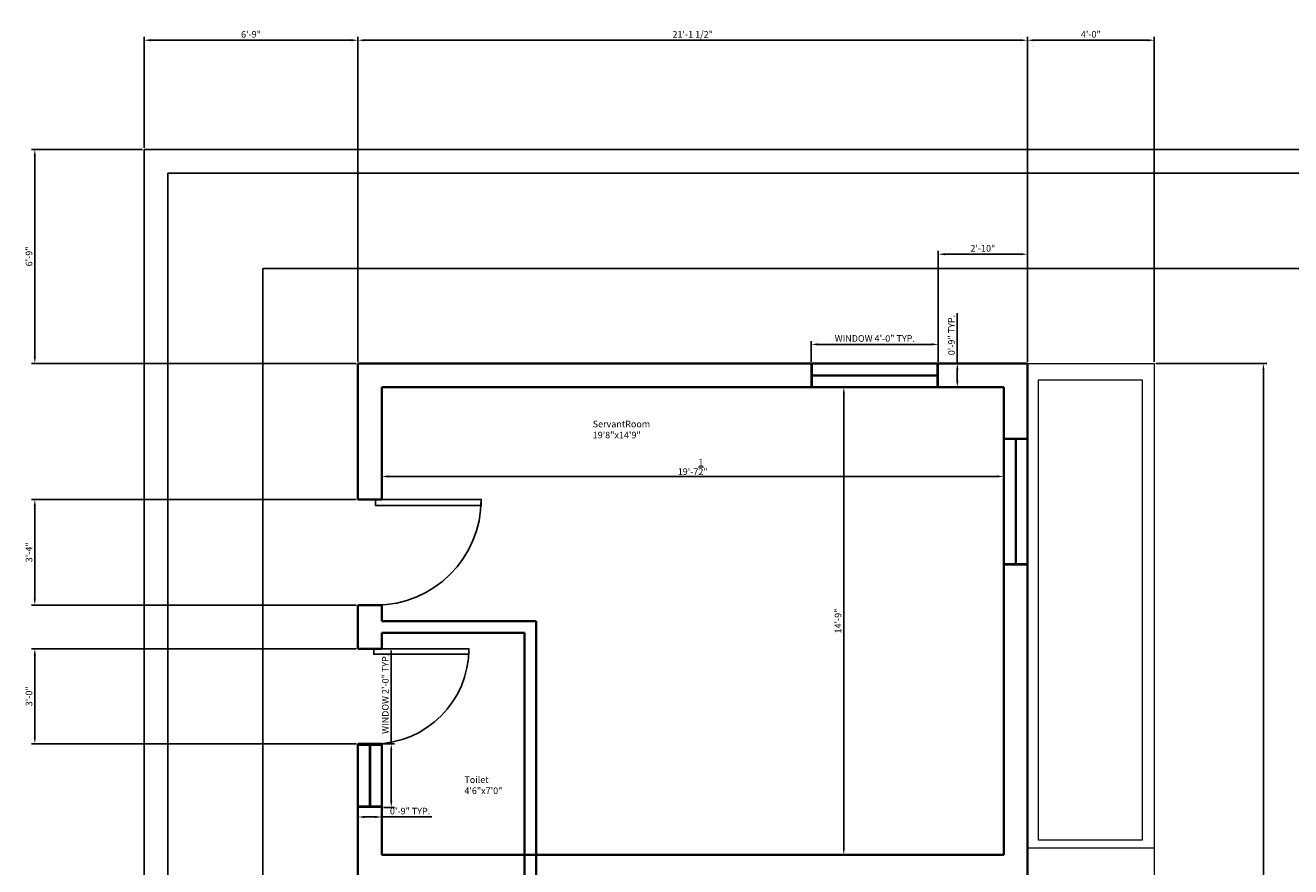
# Model space of a CAD drawing. Units: inches. Extents: x 250205121 to 250208111, y 89832590 to 89833271.
# Tile 2 of 14: x 250205121 to 250205601, y 89832953 to 89833271. Entities that reach past the tile are written whole.
import ezdxf

# ---------------------------------------------------------------- set-up
doc = ezdxf.new("R2010")
doc.units = ezdxf.units.IN
for name, color, linetype, lineweight in [('A-AREA-IDEN', 4, 'Continuous', 18), ('A-FLOR', 7, 'Continuous', 18), ('A-WALL', 7, 'Continuous', 35), ('C-PROP', 8, 'Continuous', 25), ('dimensions', 2, 'Continuous', 18), ('doors', 3, 'Continuous', 25), ('window', 4, 'Continuous', 18)]:
    doc.layers.add(name, color=color, linetype=linetype, lineweight=lineweight)
doc.styles.get("Standard").update_dxf_attribs({"font": 'arial.ttf'})
doc.dimstyles.new('ISO-25', dxfattribs={"dimtxt": 2.5, "dimasz": 2.5, "dimexe": 1.25, "dimexo": 0.625, "dimtad": 1, "dimlunit": 4, "dimtxsty": 'Standard', "dimcen": 2.5, "dimadec": 0, "dimazin": 0, "dimtfac": 1, "dimtmove": 0, "dimatfit": 3, "dimfxl": 1, "dimarcsym": 0})

# ---------------------------------------------------------------- blocks, each defined once
blk = doc.blocks.new('*U2')
for p, q in [((0, 0), (0, -5)), ((30, 0), (30, -5))]:
    blk.add_line(p, q)
blk.add_lwpolyline([(0, 0), (0, 30), (1.75, 30), (1.75, 0)], close=True)
blk.add_arc((0, 0), 30, 0, 90)
blk = doc.blocks.new('*D3')
at = {"layer": 'Defpoints', "color": 0, "transparency": 16777216}
for p in [(250205406.37, 89833134.33), (250205406.37, 89832957.33), (250205431.38, 89832957.33)]:
    blk.add_point(p, dxfattribs=at)
at = {"layer": 'dimensions', "color": 0, "lineweight": -2, "transparency": 16777216}
for p, q in [((250205406.99, 89833134.33), (250205432.63, 89833134.33)), ((250205431.38, 89833131.83), (250205431.38, 89832959.83)), ((250205406.99, 89832957.33), (250205432.63, 89832957.33))]:
    blk.add_line(p, q, dxfattribs=at)
at = {"layer": 'dimensions', "color": 0, "transparency": 16777216}
for points in [[(250205430.97, 89833131.83), (250205431.8, 89833131.83), (250205431.38, 89833134.33)], [(250205430.97, 89832959.83), (250205431.8, 89832959.83), (250205431.38, 89832957.33)]]:
    blk.add_solid(points, dxfattribs=at)
at = {"layer": 'dimensions', "color": 0, "transparency": 16777216, "insert": (250205429.48, 89833045.83), "char_height": 2.5, "attachment_point": 5, "rotation": 90}
blk.add_mtext('14\'-9"', dxfattribs=at)
blk = doc.blocks.new('*D4')
at = {"layer": 'Defpoints', "color": 0, "transparency": 16777216}
for p in [(250205256.41, 89833120.81), (250205491.91, 89833120.81), (250205491.91, 89833100.55)]:
    blk.add_point(p, dxfattribs=at)
at = {"layer": 'dimensions', "color": 0, "lineweight": -2, "transparency": 16777216}
for p, q in [((250205256.41, 89833120.18), (250205256.41, 89833099.3)), ((250205491.91, 89833120.18), (250205491.91, 89833099.3)), ((250205258.91, 89833100.55), (250205489.41, 89833100.55))]:
    blk.add_line(p, q, dxfattribs=at)
at = {"layer": 'dimensions', "color": 0, "transparency": 16777216}
for points in [[(250205258.91, 89833100.97), (250205258.91, 89833100.14), (250205256.41, 89833100.55)], [(250205489.41, 89833100.97), (250205489.41, 89833100.14), (250205491.91, 89833100.55)]]:
    blk.add_solid(points, dxfattribs=at)
at = {"layer": 'dimensions', "color": 0, "transparency": 16777216, "insert": (250205374.16, 89833104.13), "char_height": 2.5, "attachment_point": 5}
blk.add_mtext('19\'-7{\\H1x;\\S1/2;}"', dxfattribs=at)
blk = doc.blocks.new('WIN-24IN')
for p, q in [((0, 0), (0, 24.08)), ((0, 24.08), (9, 24.08)), ((9, 24.08), (9, 0)), ((0, 23.58), (9, 23.58)), ((4.3, 23.58), (4.3, 0.5)), ((4.7, 23.58), (4.7, 0.5)), ((9, 0.5), (0, 0.5)), ((9, 0), (0, 0))]:
    blk.add_line(p, q)
blk = doc.blocks.new('WIN-48IN')
for p, q in [((0, 0), (0, 48.08)), ((0, 48.08), (9, 48.08)), ((9, 48.08), (9, 0)), ((0, 47.58), (9, 47.58)), ((4.3, 47.58), (4.3, 0.5)), ((4.7, 47.58), (4.7, 0.5)), ((9, 0.5), (0, 0.5)), ((9, 0), (0, 0))]:
    blk.add_line(p, q)
blk = doc.blocks.new('*D29')
at = {"layer": 'Defpoints', "color": 0, "transparency": 16777216}
for p in [(250205256.41, 89832999.33), (250205260.02, 89832999.33), (250205256.41, 89832975.25)]:
    blk.add_point(p, dxfattribs=at)
at = {"layer": 'dimensions', "color": 0, "lineweight": -2, "transparency": 16777216}
for p, q in [((250205260.02, 89832999.33), (250205260.02, 89833034.71)), ((250205257.03, 89832999.33), (250205261.27, 89832999.33)), ((250205260.02, 89832977.75), (250205260.02, 89832996.83)), ((250205257.03, 89832975.25), (250205261.27, 89832975.25))]:
    blk.add_line(p, q, dxfattribs=at)
at = {"layer": 'dimensions', "color": 0, "transparency": 16777216}
for points in [[(250205259.6, 89832996.83), (250205260.44, 89832996.83), (250205260.02, 89832999.33)], [(250205259.6, 89832977.75), (250205260.44, 89832977.75), (250205260.02, 89832975.25)]]:
    blk.add_solid(points, dxfattribs=at)
at = {"layer": 'dimensions', "color": 0, "transparency": 16777216, "insert": (250205258.1, 89833018.27), "char_height": 2.5, "attachment_point": 5, "rotation": 90}
blk.add_mtext('WINDOW 2\'-0" TYP.', dxfattribs=at)
blk = doc.blocks.new('*D30')
at = {"layer": 'Defpoints', "color": 0, "transparency": 16777216}
for p in [(250205247.41, 89832975.25), (250205256.41, 89832975.25), (250205256.41, 89832971.64)]:
    blk.add_point(p, dxfattribs=at)
at = {"layer": 'dimensions', "color": 0, "lineweight": -2, "transparency": 16777216}
for p, q in [((250205247.41, 89832974.62), (250205247.41, 89832970.39)), ((250205256.41, 89832974.62), (250205256.41, 89832970.39)), ((250205249.91, 89832971.64), (250205253.91, 89832971.64)), ((250205256.41, 89832971.64), (250205275.4, 89832971.64))]:
    blk.add_line(p, q, dxfattribs=at)
at = {"layer": 'dimensions', "color": 0, "transparency": 16777216}
for points in [[(250205249.91, 89832972.05), (250205249.91, 89832971.22), (250205247.41, 89832971.64)], [(250205253.91, 89832972.05), (250205253.91, 89832971.22), (250205256.41, 89832971.64)]]:
    blk.add_solid(points, dxfattribs=at)
at = {"layer": 'dimensions', "color": 0, "transparency": 16777216, "insert": (250205267.15, 89832973.54), "char_height": 2.5, "attachment_point": 5}
blk.add_mtext('0\'-9" TYP.', dxfattribs=at)
blk = doc.blocks.new('*D31')
at = {"layer": 'Defpoints', "color": 0, "transparency": 16777216}
for p in [(250205419.07, 89833150.54), (250205419.07, 89833143.33), (250205467.15, 89833143.33)]:
    blk.add_point(p, dxfattribs=at)
at = {"layer": 'dimensions', "color": 0, "lineweight": -2, "transparency": 16777216}
for p, q in [((250205419.07, 89833143.95), (250205419.07, 89833151.79)), ((250205467.15, 89833143.95), (250205467.15, 89833151.79)), ((250205464.65, 89833150.54), (250205421.57, 89833150.54))]:
    blk.add_line(p, q, dxfattribs=at)
at = {"layer": 'dimensions', "color": 0, "transparency": 16777216}
for points in [[(250205421.57, 89833150.96), (250205421.57, 89833150.12), (250205419.07, 89833150.54)], [(250205464.65, 89833150.96), (250205464.65, 89833150.12), (250205467.15, 89833150.54)]]:
    blk.add_solid(points, dxfattribs=at)
at = {"layer": 'dimensions', "color": 0, "transparency": 16777216, "insert": (250205443.11, 89833152.46), "char_height": 2.5, "attachment_point": 5, "rotation": 0}
blk.add_mtext('WINDOW 4\'-0" TYP.', dxfattribs=at)
blk = doc.blocks.new('*D32')
at = {"layer": 'Defpoints', "color": 0, "transparency": 16777216}
for p in [(250205467.15, 89833143.33), (250205474.36, 89833143.33), (250205467.15, 89833134.33)]:
    blk.add_point(p, dxfattribs=at)
at = {"layer": 'dimensions', "color": 0, "lineweight": -2, "transparency": 16777216}
for p, q in [((250205474.36, 89833143.33), (250205474.36, 89833162.32)), ((250205467.77, 89833143.33), (250205475.61, 89833143.33)), ((250205474.36, 89833136.83), (250205474.36, 89833140.83)), ((250205467.77, 89833134.33), (250205475.61, 89833134.33))]:
    blk.add_line(p, q, dxfattribs=at)
at = {"layer": 'dimensions', "color": 0, "transparency": 16777216}
for points in [[(250205473.94, 89833140.83), (250205474.78, 89833140.83), (250205474.36, 89833143.33)], [(250205473.94, 89833136.83), (250205474.78, 89833136.83), (250205474.36, 89833134.33)]]:
    blk.add_solid(points, dxfattribs=at)
at = {"layer": 'dimensions', "color": 0, "transparency": 16777216, "insert": (250205472.46, 89833154.07), "char_height": 2.5, "attachment_point": 5, "rotation": 90}
blk.add_mtext('0\'-9" TYP.', dxfattribs=at)
blk = doc.blocks.new('*D43')
at = {"layer": 'Defpoints', "color": 0, "transparency": 16777216}
for p in [(250205247.41, 89833265.68), (250205166.41, 89833224.33), (250205247.41, 89833143.33)]:
    blk.add_point(p, dxfattribs=at)
at = {"layer": 'dimensions', "color": 0, "lineweight": -2, "transparency": 16777216}
for p, q in [((250205166.41, 89833224.95), (250205166.41, 89833266.93)), ((250205247.41, 89833143.95), (250205247.41, 89833266.93)), ((250205168.91, 89833265.68), (250205244.91, 89833265.68))]:
    blk.add_line(p, q, dxfattribs=at)
at = {"layer": 'dimensions', "color": 0, "transparency": 16777216}
for points in [[(250205168.91, 89833266.09), (250205168.91, 89833265.26), (250205166.41, 89833265.68)], [(250205244.91, 89833266.09), (250205244.91, 89833265.26), (250205247.41, 89833265.68)]]:
    blk.add_solid(points, dxfattribs=at)
at = {"layer": 'dimensions', "color": 0, "transparency": 16777216, "insert": (250205206.91, 89833267.58), "char_height": 2.5, "attachment_point": 5}
blk.add_mtext('6\'-9"', dxfattribs=at)
blk = doc.blocks.new('*D44')
at = {"layer": 'Defpoints', "color": 0, "transparency": 16777216}
for p in [(250205125.06, 89833224.33), (250205166.41, 89833224.33), (250205247.41, 89833143.33)]:
    blk.add_point(p, dxfattribs=at)
at = {"layer": 'dimensions', "color": 0, "lineweight": -2, "transparency": 16777216}
for p, q in [((250205165.78, 89833224.33), (250205123.81, 89833224.33)), ((250205125.06, 89833145.83), (250205125.06, 89833221.83)), ((250205246.78, 89833143.33), (250205123.81, 89833143.33))]:
    blk.add_line(p, q, dxfattribs=at)
at = {"layer": 'dimensions', "color": 0, "transparency": 16777216}
for points in [[(250205124.64, 89833221.83), (250205125.47, 89833221.83), (250205125.06, 89833224.33)], [(250205124.64, 89833145.83), (250205125.47, 89833145.83), (250205125.06, 89833143.33)]]:
    blk.add_solid(points, dxfattribs=at)
at = {"layer": 'dimensions', "color": 0, "transparency": 16777216, "insert": (250205123.16, 89833183.83), "char_height": 2.5, "attachment_point": 5, "rotation": 90}
blk.add_mtext('6\'-9"', dxfattribs=at)
blk = doc.blocks.new('*D45')
at = {"layer": 'Defpoints', "color": 0, "transparency": 16777216}
for p in [(250205500.91, 89833265.68), (250205247.41, 89833143.33), (250205500.91, 89833143.33)]:
    blk.add_point(p, dxfattribs=at)
at = {"layer": 'dimensions', "color": 0, "lineweight": -2, "transparency": 16777216}
for p, q in [((250205247.41, 89833143.95), (250205247.41, 89833266.93)), ((250205500.91, 89833143.95), (250205500.91, 89833266.93)), ((250205249.91, 89833265.68), (250205498.41, 89833265.68))]:
    blk.add_line(p, q, dxfattribs=at)
at = {"layer": 'dimensions', "color": 0, "transparency": 16777216}
for points in [[(250205249.91, 89833266.09), (250205249.91, 89833265.26), (250205247.41, 89833265.68)], [(250205498.41, 89833266.09), (250205498.41, 89833265.26), (250205500.91, 89833265.68)]]:
    blk.add_solid(points, dxfattribs=at)
at = {"layer": 'dimensions', "color": 0, "transparency": 16777216, "insert": (250205374.16, 89833267.6), "char_height": 2.5, "attachment_point": 5}
blk.add_mtext('21\'-1 1/2"', dxfattribs=at)
blk = doc.blocks.new('*D46')
at = {"layer": 'Defpoints', "color": 0, "transparency": 16777216}
for p in [(250205548.91, 89833265.68), (250205500.91, 89833143.33), (250205548.91, 89833143.33)]:
    blk.add_point(p, dxfattribs=at)
at = {"layer": 'dimensions', "color": 0, "lineweight": -2, "transparency": 16777216}
for p, q in [((250205500.91, 89833143.95), (250205500.91, 89833266.93)), ((250205548.91, 89833143.95), (250205548.91, 89833266.93)), ((250205503.41, 89833265.68), (250205546.41, 89833265.68))]:
    blk.add_line(p, q, dxfattribs=at)
at = {"layer": 'dimensions', "color": 0, "transparency": 16777216}
for points in [[(250205503.41, 89833266.09), (250205503.41, 89833265.26), (250205500.91, 89833265.68)], [(250205546.41, 89833266.09), (250205546.41, 89833265.26), (250205548.91, 89833265.68)]]:
    blk.add_solid(points, dxfattribs=at)
at = {"layer": 'dimensions', "color": 0, "transparency": 16777216, "insert": (250205524.91, 89833267.58), "char_height": 2.5, "attachment_point": 5}
blk.add_mtext('4\'-0"', dxfattribs=at)
blk = doc.blocks.new('*D48')
at = {"layer": 'Defpoints', "color": 0, "transparency": 16777216}
for p in [(250205548.91, 89833143.33), (250205548.91, 89832714.33), (250205590.26, 89832714.33)]:
    blk.add_point(p, dxfattribs=at)
at = {"layer": 'dimensions', "color": 0, "lineweight": -2, "transparency": 16777216}
for p, q in [((250205549.53, 89833143.33), (250205591.51, 89833143.33)), ((250205590.26, 89833140.83), (250205590.26, 89832716.83)), ((250205549.53, 89832714.33), (250205591.51, 89832714.33))]:
    blk.add_line(p, q, dxfattribs=at)
at = {"layer": 'dimensions', "color": 0, "transparency": 16777216}
for points in [[(250205589.84, 89833140.83), (250205590.67, 89833140.83), (250205590.26, 89833143.33)], [(250205589.84, 89832716.83), (250205590.67, 89832716.83), (250205590.26, 89832714.33)]]:
    blk.add_solid(points, dxfattribs=at)
at = {"layer": 'dimensions', "color": 0, "transparency": 16777216, "insert": (250205588.36, 89832928.83), "char_height": 2.5, "attachment_point": 5, "rotation": 90}
blk.add_mtext('35\'-9"', dxfattribs=at)
blk = doc.blocks.new('*D50')
at = {"layer": 'Defpoints', "color": 0, "transparency": 16777216}
for p in [(250205125.06, 89833091.83), (250205247.41, 89833091.83), (250205247.41, 89833051.83)]:
    blk.add_point(p, dxfattribs=at)
at = {"layer": 'dimensions', "color": 0, "lineweight": -2, "transparency": 16777216}
for p, q in [((250205246.78, 89833091.83), (250205123.81, 89833091.83)), ((250205125.06, 89833054.33), (250205125.06, 89833089.33)), ((250205246.78, 89833051.83), (250205123.81, 89833051.83))]:
    blk.add_line(p, q, dxfattribs=at)
at = {"layer": 'dimensions', "color": 0, "transparency": 16777216}
for points in [[(250205124.64, 89833089.33), (250205125.47, 89833089.33), (250205125.06, 89833091.83)], [(250205124.64, 89833054.33), (250205125.47, 89833054.33), (250205125.06, 89833051.83)]]:
    blk.add_solid(points, dxfattribs=at)
at = {"layer": 'dimensions', "color": 0, "transparency": 16777216, "insert": (250205123.16, 89833071.83), "char_height": 2.5, "attachment_point": 5, "rotation": 90}
blk.add_mtext('3\'-4"', dxfattribs=at)
blk = doc.blocks.new('*D51')
at = {"layer": 'Defpoints', "color": 0, "transparency": 16777216}
for p in [(250205125.06, 89833035.33), (250205247.41, 89833035.33), (250205247.41, 89832999.33)]:
    blk.add_point(p, dxfattribs=at)
at = {"layer": 'dimensions', "color": 0, "lineweight": -2, "transparency": 16777216}
for p, q in [((250205246.78, 89833035.33), (250205123.81, 89833035.33)), ((250205125.06, 89833001.83), (250205125.06, 89833032.83)), ((250205246.78, 89832999.33), (250205123.81, 89832999.33))]:
    blk.add_line(p, q, dxfattribs=at)
at = {"layer": 'dimensions', "color": 0, "transparency": 16777216}
for points in [[(250205124.64, 89833032.83), (250205125.47, 89833032.83), (250205125.06, 89833035.33)], [(250205124.64, 89833001.83), (250205125.47, 89833001.83), (250205125.06, 89832999.33)]]:
    blk.add_solid(points, dxfattribs=at)
at = {"layer": 'dimensions', "color": 0, "transparency": 16777216, "insert": (250205123.16, 89833017.33), "char_height": 2.5, "attachment_point": 5, "rotation": 90}
blk.add_mtext('3\'-0"', dxfattribs=at)
blk = doc.blocks.new('*D53')
at = {"layer": 'Defpoints', "color": 0, "transparency": 16777216}
for p in [(250205500.91, 89833184.68), (250205467.15, 89833143.33), (250205500.91, 89833143.33)]:
    blk.add_point(p, dxfattribs=at)
at = {"layer": 'dimensions', "color": 0, "lineweight": -2, "transparency": 16777216}
for p, q in [((250205467.15, 89833143.95), (250205467.15, 89833185.93)), ((250205469.65, 89833184.68), (250205498.41, 89833184.68)), ((250205500.91, 89833143.95), (250205500.91, 89833185.93))]:
    blk.add_line(p, q, dxfattribs=at)
at = {"layer": 'dimensions', "color": 0, "transparency": 16777216}
for points in [[(250205469.65, 89833185.09), (250205469.65, 89833184.26), (250205467.15, 89833184.68)], [(250205498.41, 89833185.09), (250205498.41, 89833184.26), (250205500.91, 89833184.68)]]:
    blk.add_solid(points, dxfattribs=at)
at = {"layer": 'dimensions', "color": 0, "transparency": 16777216, "insert": (250205484.03, 89833186.58), "char_height": 2.5, "attachment_point": 5}
blk.add_mtext('2\'-10"', dxfattribs=at)

msp = doc.modelspace()

# ---------------------------------------------------------------- linework, layer by layer
at = {"layer": 'A-FLOR'}
for p, q in [((250205500.908, 89833143.328), (250205524.908, 89833143.328)), ((250205524.908, 89833143.328), (250205548.908, 89833143.328)), ((250205548.908, 89833143.328), (250205548.908, 89832714.328)), ((250205500.908, 89832959.99), (250205548.908, 89832959.99))]:
    msp.add_line(p, q, dxfattribs=at)
msp.add_lwpolyline([(250205505.113, 89833137.184), (250205544.324, 89833137.184), (250205544.324, 89832962.894), (250205505.113, 89832962.894)], close=True, dxfattribs=at)
at = {"layer": 'A-WALL'}
for p, q in [((250205256.408, 89833143.328), (250205247.408, 89833143.328)), ((250205247.408, 89833143.328), (250205247.408, 89833134.328)), ((250205500.908, 89833143.328), (250205256.408, 89833143.328)), ((250205500.908, 89833134.328), (250205500.908, 89833143.328)), ((250205247.408, 89833134.328), (250205247.408, 89833091.828)), ((250205256.408, 89833134.328), (250205491.908, 89833134.328)), ((250205256.408, 89833134.328), (250205256.408, 89833091.828)), ((250205491.908, 89832957.328), (250205491.908, 89833134.328)), ((250205500.908, 89832948.328), (250205500.908, 89833134.328)), ((250205247.408, 89833091.828), (250205256.408, 89833091.828)), ((250205256.408, 89833051.828), (250205247.408, 89833051.828)), ((250205247.408, 89833051.828), (250205247.408, 89833035.328)), ((250205256.408, 89833045.828), (250205256.408, 89833051.828)), ((250205256.408, 89833051.828), (250205256.408, 89833045.828)), ((250205256.408, 89833045.828), (250205314.908, 89833045.828)), ((250205314.908, 89833045.828), (250205314.908, 89832888.328)), ((250205256.408, 89833041.328), (250205310.408, 89833041.328)), ((250205256.408, 89833041.328), (250205256.408, 89833035.328)), ((250205256.408, 89833041.328), (250205256.408, 89833035.328)), ((250205310.408, 89833041.328), (250205310.408, 89832888.328)), ((250205256.408, 89833035.328), (250205247.408, 89833035.328)), ((250205247.408, 89832999.328), (250205256.408, 89832999.328)), ((250205247.408, 89832999.328), (250205247.408, 89832948.328)), ((250205256.408, 89832999.328), (250205256.408, 89832957.328)), ((250205256.408, 89832957.328), (250205491.908, 89832957.328))]:
    msp.add_line(p, q, dxfattribs=at)
at = {"layer": 'C-PROP'}
for p, q in [((250205166.408, 89833224.328), (250205166.408, 89832633.328)), ((250205500.908, 89833224.328), (250205166.408, 89833224.328)), ((250205500.908, 89833224.328), (250205977.908, 89833224.328)), ((250205500.908, 89833215.328), (250205175.408, 89833215.328)), ((250205175.408, 89833215.328), (250205175.408, 89832642.328)), ((250205977.908, 89833215.328), (250205500.908, 89833215.328)), ((250205500.908, 89833179.328), (250205211.408, 89833179.328)), ((250205211.408, 89833179.328), (250205211.408, 89832678.328)), ((250205500.908, 89833179.328), (250205509.908, 89833179.328)), ((250205509.908, 89833179.328), (250205680.908, 89833179.328))]:
    msp.add_line(p, q, dxfattribs=at)

# ---------------------------------------------------------------- block references
at = {"layer": 'doors', "rotation": 270}
for p, xscale, yscale, zscale in [((250205254.074, 89833091.828), 1.333333333333333, 1.333333333333333, 1.333333333333333), ((250205253.408, 89833035.328), 1.199999999999999, 1.199999999999999, 1.199999999999999)]:
    msp.add_blockref('*U2', p, dxfattribs=dict(at, xscale=xscale, yscale=yscale, zscale=zscale))
at = {"layer": 'window', "rotation": 90.00000004715952}
msp.add_blockref('WIN-48IN', (250205467.149, 89833134.328), dxfattribs=at)
at = {"layer": 'window'}
for name, p in [('WIN-48IN', (250205491.908, 89833067.021)), ('WIN-24IN', (250205247.408, 89832975.249))]:
    msp.add_blockref(name, p, dxfattribs=at)

# ---------------------------------------------------------------- texts
at = {"layer": 'A-AREA-IDEN', "char_height": 2.5, "attachment_point": 1}
for s, insert in [('ServantRoom\\P19\'8"x14\'9"', (250205336.292, 89833121.638)), ('Toilet\\P4\'6"x7\'0"', (250205287.708, 89832986.993))]:
    msp.add_mtext_dynamic_manual_height_columns(s, width=2.73747, gutter_width=12.5, heights=[0], dxfattribs=dict(at, insert=insert))

# ---------------------------------------------------------------- dimensions: what is measured, and where the dimension line sits
at = {"layer": 'dimensions'}
for base, p1, p2, override, picture, middle in [((250205500.908, 89833265.678), (250205247.408, 89833143.328), (250205500.908, 89833143.328), {"dimdec": 1, "dimlfac": 1, "dimrnd": 0, "dimzin": 1, "dimdsep": 46, "dimlunit": 4, "dimfrac": 2}, '*D45', (250205374.158, 89833267.596)), ((250205247.408, 89833265.678), (250205166.408, 89833224.328), (250205247.408, 89833143.328), {"dimdec": 1, "dimlfac": 1, "dimrnd": 0, "dimzin": 1, "dimdsep": 46, "dimlunit": 4, "dimfrac": 2}, '*D43', (250205206.908, 89833267.579)), ((250205548.908, 89833265.678), (250205500.908, 89833143.328), (250205548.908, 89833143.328), {"dimdec": 1, "dimlfac": 1, "dimrnd": 0, "dimzin": 1, "dimdsep": 46, "dimlunit": 4, "dimfrac": 2}, '*D46', (250205524.908, 89833267.579)), ((250205491.908, 89833100.553), (250205256.408, 89833120.808), (250205491.908, 89833120.808), {"dimclrd": 0, "dimclre": 0, "dimclrt": 0}, '*D4', (250205374.158, 89833104.126))]:
    dim = msp.add_linear_dim(base=base, p1=p1, p2=p2, dimstyle='ISO-25', override=override, dxfattribs=at)
    dim.commit()
    dim.dimension.update_dxf_attribs({"geometry": picture, "text_midpoint": middle})
for base, p1, p2, angle, override, picture, middle in [((250205125.058, 89833224.328), (250205247.408, 89833143.328), (250205166.408, 89833224.328), 90, {"dimdec": 1, "dimlfac": 1, "dimrnd": 0, "dimzin": 1, "dimdsep": 46, "dimlunit": 4, "dimfrac": 2}, '*D44', (250205123.156, 89833183.828)), ((250205500.908, 89833184.678), (250205467.149, 89833143.328), (250205500.908, 89833143.328), 360, {"dimdec": 1, "dimlfac": 1, "dimrnd": 0, "dimzin": 1, "dimdsep": 46, "dimlunit": 4, "dimfrac": 2}, '*D53', (250205484.029, 89833186.579)), ((250205590.258, 89832714.328), (250205548.908, 89833143.328), (250205548.908, 89832714.328), 270, {"dimdec": 1, "dimlfac": 1, "dimrnd": 0, "dimzin": 1, "dimdsep": 46, "dimlunit": 4, "dimfrac": 2}, '*D48', (250205588.355, 89832928.828)), ((250205431.382, 89832957.328), (250205406.369, 89833134.328), (250205406.369, 89832957.328), 90, {"dimclrd": 0, "dimclre": 0, "dimclrt": 0}, '*D3', (250205429.481, 89833045.828)), ((250205125.058, 89833091.828), (250205247.408, 89833051.828), (250205247.408, 89833091.828), 90, {"dimdec": 1, "dimlfac": 1, "dimrnd": 0, "dimzin": 1, "dimdsep": 46, "dimlunit": 4, "dimfrac": 2}, '*D50', (250205123.155, 89833071.828)), ((250205125.058, 89833035.328), (250205247.408, 89832999.328), (250205247.408, 89833035.328), 90, {"dimdec": 1, "dimlfac": 1, "dimrnd": 0, "dimzin": 1, "dimdsep": 46, "dimlunit": 4, "dimfrac": 2}, '*D51', (250205123.155, 89833017.328))]:
    dim = msp.add_linear_dim(base=base, p1=p1, p2=p2, angle=angle, dimstyle='ISO-25', override=override, dxfattribs=at)
    dim.commit()
    dim.dimension.update_dxf_attribs({"geometry": picture, "text_midpoint": middle})
for base, p1, p2, angle, text, picture, middle in [((250205474.361, 89833143.328), (250205467.149, 89833134.328), (250205467.149, 89833143.328), 90, '<> TYP.', '*D32', (250205472.46, 89833154.072)), ((250205419.071, 89833150.54), (250205467.149, 89833143.328), (250205419.071, 89833143.328), 180, 'WINDOW <> TYP.', '*D31', (250205443.11, 89833152.458)), ((250205260.019, 89832999.328), (250205256.408, 89832975.249), (250205256.408, 89832999.328), 90, 'WINDOW <> TYP.', '*D29', (250205258.101, 89833018.271))]:
    dim = msp.add_linear_dim(base=base, p1=p1, p2=p2, angle=angle, text=text, dimstyle='ISO-25', override={"dimdec": 1, "dimlfac": 1, "dimrnd": 0, "dimzin": 1, "dimdsep": 46, "dimlunit": 4, "dimfrac": 2}, dxfattribs=at)
    dim.commit()
    dim.dimension.update_dxf_attribs({"geometry": picture, "text_midpoint": middle})
dim = msp.add_linear_dim(base=(250205256.408, 89832971.637), p1=(250205247.408, 89832975.249), p2=(250205256.408, 89832975.249), text='<> TYP.', dimstyle='ISO-25', override={"dimdec": 1, "dimlfac": 1, "dimrnd": 0, "dimzin": 1, "dimdsep": 46, "dimlunit": 4, "dimfrac": 2}, dxfattribs=at)
dim.commit()
dim.dimension.update_dxf_attribs({"geometry": '*D30', "text_midpoint": (250205267.152, 89832973.539)})

doc.saveas('drawing.dxf')
